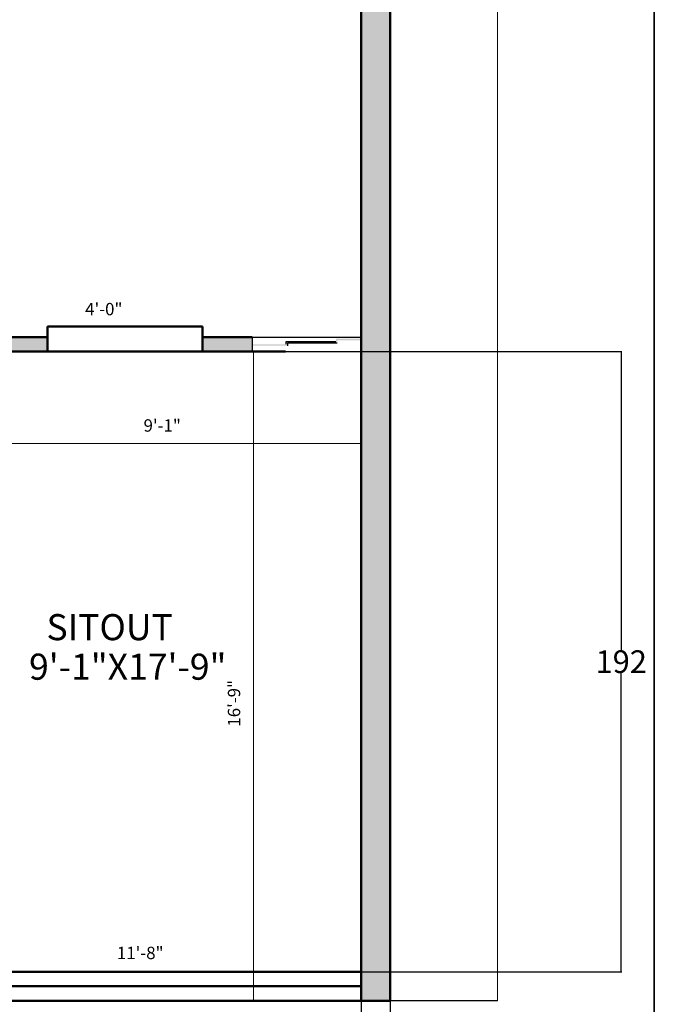
# Model space of a CAD drawing. Units: inches. Extents: x 1381 to 2246, y 1317 to 2168.
# Tile 12 of 15: x 2048 to 2244, y 1471 to 1776. Entities that reach past the tile are written whole.
import ezdxf

# ---------------------------------------------------------------- set-up
doc = ezdxf.new("R2010")
doc.units = ezdxf.units.IN
doc.header["$MEASUREMENT"] = 0
for name, color, linetype, lineweight in [('A-ANNO-DIMS', 2, 'Continuous', 18), ('A-ANNO-TEXT', 7, 'Continuous', 18), ('A-ANNO-TTLB', 7, 'Continuous', 35), ('A-AREA-IDEN', 3, 'Continuous', 25), ('A-GLAZ', 4, 'Continuous', 25), ('A-WALL', 7, 'Continuous', 50), ('A-WALL-PATT', 8, 'Continuous', 13)]:
    doc.layers.add(name, color=color, linetype=linetype, lineweight=lineweight)
doc.styles.get("Standard").update_dxf_attribs({"font": 'arial.ttf'})
doc.dimstyles.get("Standard").update_dxf_attribs({"dimtxt": 7, "dimasz": 0.18, "dimexe": 0.18, "dimexo": 0.0625, "dimgap": 0.09, "dimtad": 0, "dimtih": 1, "dimtoh": 1, "dimdec": 1, "dimzin": 0, "dimdsep": 46, "dimlunit": 3, "dimtxsty": 'Standard', "dimcen": 0.09, "dimadec": 0, "dimazin": 0, "dimtfac": 1, "dimtdec": 1, "dimtofl": 0, "dimtmove": 0, "dimatfit": 3, "dimfxl": 1, "dimtolj": 1, "dimtzin": 0, "dimarcsym": 0})

# ---------------------------------------------------------------- blocks, each defined once
blk = doc.blocks.new('*D75')
at = {"layer": 'A-ANNO-DIMS', "color": 0, "lineweight": -2, "transparency": 16777216}
for p, q in [((1862.81, 1471.85), (1862.81, 1384.36)), ((2162.31, 1471.85), (2162.31, 1384.36)), ((1862.99, 1384.54), (2000.57, 1384.54)), ((2162.13, 1384.54), (2024.54, 1384.54))]:
    blk.add_line(p, q, dxfattribs=at)
at = {"layer": 'A-ANNO-DIMS', "color": 0, "transparency": 16777216}
for points in [[(1862.99, 1384.57), (1862.99, 1384.51), (1862.81, 1384.54)], [(2162.13, 1384.57), (2162.13, 1384.51), (2162.31, 1384.54)]]:
    blk.add_solid(points, dxfattribs=at)
at = {"layer": 'Defpoints', "color": 0, "transparency": 16777216}
for p in [(1862.81, 1471.92), (2162.31, 1471.92), (2162.31, 1384.54)]:
    blk.add_point(p, dxfattribs=at)
at = {"layer": 'A-ANNO-DIMS', "color": 0, "transparency": 16777216, "insert": (2012.56, 1384.54), "char_height": 7, "attachment_point": 5}
blk.add_mtext('\\A1;299.5', dxfattribs=at)
blk = doc.blocks.new('*D86')
at = {"layer": 'A-ANNO-DIMS', "color": 0, "lineweight": -2, "transparency": 16777216}
for p, q in [((2153.37, 1672.92), (2234.02, 1672.92)), ((2233.84, 1672.74), (2233.84, 1580.58)), ((2233.84, 1481.1), (2233.84, 1573.25)), ((2153.37, 1480.92), (2234.02, 1480.92))]:
    blk.add_line(p, q, dxfattribs=at)
at = {"layer": 'A-ANNO-DIMS', "color": 0, "transparency": 16777216}
for points in [[(2233.81, 1672.74), (2233.87, 1672.74), (2233.84, 1672.92)], [(2233.81, 1481.1), (2233.87, 1481.1), (2233.84, 1480.92)]]:
    blk.add_solid(points, dxfattribs=at)
at = {"layer": 'Defpoints', "color": 0, "transparency": 16777216}
for p in [(2153.31, 1672.92), (2233.84, 1672.92), (2153.31, 1480.92)]:
    blk.add_point(p, dxfattribs=at)
at = {"layer": 'A-ANNO-DIMS', "color": 0, "transparency": 16777216, "insert": (2233.84, 1576.92), "char_height": 7, "attachment_point": 5}
blk.add_mtext('\\A1;192', dxfattribs=at)
blk = doc.blocks.new('*D91')
at = {"layer": 'A-ANNO-DIMS', "color": 0, "lineweight": -2, "transparency": 16777216}
for p, q in [((2012.56, 1471.85), (2012.56, 1384.36)), ((2153.31, 1471.85), (2153.31, 1384.36)), ((2012.74, 1384.54), (2068.61, 1384.54)), ((2153.13, 1384.54), (2097.25, 1384.54))]:
    blk.add_line(p, q, dxfattribs=at)
at = {"layer": 'A-ANNO-DIMS', "color": 0, "transparency": 16777216}
for points in [[(2012.74, 1384.57), (2012.74, 1384.51), (2012.56, 1384.54)], [(2153.13, 1384.57), (2153.13, 1384.51), (2153.31, 1384.54)]]:
    blk.add_solid(points, dxfattribs=at)
at = {"layer": 'Defpoints', "color": 0, "transparency": 16777216}
for p in [(2012.56, 1471.92), (2153.31, 1471.92), (2153.31, 1384.54)]:
    blk.add_point(p, dxfattribs=at)
at = {"layer": 'A-ANNO-DIMS', "color": 0, "transparency": 16777216, "insert": (2082.93, 1384.54), "char_height": 7, "attachment_point": 5}
blk.add_mtext('\\A1;140.75', dxfattribs=at)

msp = doc.modelspace()

# ---------------------------------------------------------------- hatches: boundary and pattern name
at = {"layer": 'A-GLAZ'}
h = msp.add_hatch(color=256, dxfattribs=at)
h.dxf.hatch_style = 1
h.paths.add_polyline_path([(2130.6579, 1675.6607), (2145.9627, 1675.6607), (2145.9627, 1676.3635), (2153.3052, 1676.3635), (2153.3052, 1676.9597), (2145.5577, 1676.9597), (2145.5577, 1676.0866), (2130.125, 1676.0866), (2130.125, 1675.1663), (2119.6192, 1675.1663), (2119.6192, 1674.7024), (2130.6579, 1674.7024)])
at = {"layer": 'A-WALL-PATT'}
h = msp.add_hatch(color=256, dxfattribs=at)
h.dxf.hatch_style = 1
h.paths.add_polyline_path([(1990.4785, 1915.9163), (1929.807, 1915.9163), (1929.807, 1911.4163), (1990.4785, 1911.4163)], flags=17)
h.paths.add_polyline_path([(1900.7902, 1915.9163), (1871.8052, 1915.9163), (1871.8052, 1911.4163), (1900.7902, 1911.4163)], flags=17)
h.paths.add_polyline_path([(2043.2216, 1915.9163), (2038.3052, 1915.9163), (2038.3052, 2035.4163), (2098.0373, 2035.4163), (2098.0373, 2039.9163), (2033.8052, 2039.9163), (2033.8052, 1915.9163), (2028.7731, 1915.9163), (2028.7731, 1911.4163), (2043.2216, 1911.4163)], flags=17)
h.paths.add_polyline_path([(2153.3052, 1915.9163), (2085.2216, 1915.9163), (2085.2216, 1911.4163), (2153.3052, 1911.4163)], flags=17)
h.paths.add_polyline_path([(1935.508, 1911.4163), (1931.008, 1911.4163), (1931.008, 1779.4163), (1899.8394, 1779.4163), (1899.8394, 1774.9163), (1902.8052, 1774.9163), (1979.3052, 1774.9163), (1979.3052, 1770.3401), (1983.8052, 1770.3401), (1983.8052, 1779.4163), (1935.508, 1779.4163)], flags=17)
h.paths.add_polyline_path([(1871.8052, 2083.9163), (2153.3052, 2083.9163), (2153.3052, 2039.9163), (2141.7178, 2039.9163), (2141.7178, 2035.4163), (2153.3052, 2035.4163), (2153.3052, 1471.9163), (2162.3052, 1471.9163), (2162.3052, 2092.9163), (1862.8052, 2092.9163), (1862.8052, 1471.9163), (1904.4174, 1471.9163), (1904.4174, 1480.9163), (1871.8052, 1480.9163), (1871.8052, 1569.4163), (1964.2348, 1569.4163), (1964.2348, 1578.4163), (1871.8052, 1578.4163)])
h.paths.add_polyline_path([(1907.3052, 1729.193), (1902.8052, 1729.193), (1902.8052, 1714.9163), (1871.8052, 1714.9163), (1871.8052, 1710.4163), (1932.8736, 1710.4163), (1932.8736, 1714.9163), (1907.3052, 1714.9163)], flags=17)
h.paths.add_polyline_path([(2044.3052, 1644.4163), (2039.8052, 1644.4163), (2039.8052, 1618.2205), (2044.3052, 1618.2205)], flags=17)
h.paths.add_polyline_path([(2044.3052, 1581.7679), (2039.8052, 1581.7679), (2039.8052, 1578.4163), (2027.577, 1578.4163), (2027.577, 1569.4163), (2044.3052, 1569.4163)], flags=17)
h = msp.add_hatch(color=256, dxfattribs=at)
h.dxf.hatch_style = 1
h.paths.add_polyline_path([(1873.9195, 1779.4163), (1871.8052, 1779.4163), (1871.8052, 1774.9163), (1873.9195, 1774.9163)])
h.paths.add_polyline_path([(1983.8052, 1779.4163), (1935.508, 1779.4163), (1935.508, 1911.4163), (1931.008, 1911.4163), (1931.008, 1779.4163), (1899.8394, 1779.4163), (1899.8394, 1774.9163), (1902.8052, 1774.9163), (1979.3052, 1774.9163), (1979.3052, 1770.3401), (1983.8052, 1770.3401)])
h.paths.add_polyline_path([(1907.3052, 1774.9163), (1902.8052, 1774.9163), (1902.8052, 1755.1129), (1907.3052, 1755.1129)])
h.paths.add_polyline_path([(1983.8052, 1734.7997), (1979.3052, 1734.7997), (1979.3052, 1714.9163), (1973.3503, 1714.9163), (1973.3503, 1710.4163), (1983.8052, 1710.4163)])
h.paths.add_polyline_path([(2044.3052, 1732.454), (2039.8052, 1732.454), (2039.8052, 1716.0149), (2024.8052, 1716.0149), (2024.8052, 1710.4163), (2039.8052, 1710.4163), (2039.8052, 1644.4163), (2044.3052, 1644.4163)])
h.paths.add_polyline_path([(2056.2659, 1677.4163), (2044.3052, 1677.4163), (2044.3052, 1672.9163), (2056.2659, 1672.9163)])
h.paths.add_polyline_path([(2119.6192, 1677.4163), (2104.2659, 1677.4163), (2104.2659, 1672.9163), (2119.6192, 1672.9163)])
h.paths.add_polyline_path([(2012.5552, 1480.9163), (1952.401, 1480.9163), (1952.401, 1471.9163), (2012.5552, 1471.9163)])
h.paths.add_polyline_path([(1870.8149, 1834.6368), (1933.6567, 1834.6368), (1933.6567, 1847.0047), (1870.8149, 1847.0047)], flags=9)

# ---------------------------------------------------------------- linework, layer by layer
at = {"layer": 'A-ANNO-DIMS'}
for p, q in [((2195.5946, 2092.9163), (2195.5946, 1471.9163)), ((2120.0865, 1471.9163), (2120.0865, 1672.9163)), ((2039.8052, 1644.4163), (2153.3052, 1644.4163))]:
    msp.add_line(p, q, dxfattribs=at)
at = {"layer": 'A-ANNO-TTLB'}
msp.add_line((2244.072, 2167.8236), (2244.072, 1316.7761), dxfattribs=at)
at = {"layer": 'A-GLAZ'}
for p, q in [((2119.6192, 1677.4163), (2119.6192, 1672.9163)), ((2119.6192, 1677.4163), (2153.3052, 1677.4163)), ((2153.3052, 1672.9163), (2153.3052, 1677.4163)), ((2130.125, 1675.1663), (2130.125, 1676.0866)), ((2130.125, 1676.0866), (2145.5577, 1676.0866)), ((2130.6579, 1674.7024), (2130.6579, 1675.6607)), ((2130.6579, 1675.6607), (2145.9627, 1675.6607)), ((2119.6192, 1672.9163), (2153.3052, 1672.9163)), ((2195.5946, 1471.9163), (2162.3052, 1471.9163))]:
    msp.add_line(p, q, dxfattribs=at)
at = {"layer": 'A-WALL'}
for p, q in [((2162.3052, 2092.9163), (2162.3052, 1471.9163)), ((2153.3052, 2035.4163), (2153.3052, 1471.9163)), ((2056.2659, 1672.9163), (2056.2659, 1680.6861)), ((2056.2659, 1680.6861), (2104.2659, 1680.6861)), ((2104.2659, 1680.6861), (2104.2659, 1672.9163)), ((2044.3052, 1677.4163), (2056.2659, 1677.4163)), ((2104.2659, 1677.4163), (2119.6192, 1677.4163)), ((2044.3052, 1672.9163), (2129.9278, 1672.9163)), ((1871.8052, 1480.9163), (2153.3052, 1480.9163)), ((2012.5552, 1480.9163), (2153.3052, 1480.9163)), ((2153.3052, 1480.9163), (2153.3052, 1471.9163)), ((2012.5552, 1476.4163), (2153.3052, 1476.4163)), ((1862.8052, 1471.9163), (2162.3052, 1471.9163)), ((2153.3052, 1471.9163), (2012.5552, 1471.9163))]:
    msp.add_line(p, q, dxfattribs=at)

# ---------------------------------------------------------------- texts
at = {"layer": 'A-ANNO-TEXT'}
for s, p in [('4\'-0"', (2067.9384, 1684.1577)), ('9\'-1"', (2086.0202, 1648.1237)), ('11\'-8"', (2077.7577, 1484.8192))]:
    msp.add_text(s, height=3.83139, dxfattribs=at).set_placement(p)
msp.add_text('16\'-9"', height=3.83139, rotation=90, dxfattribs=at).set_placement((2115.9259, 1556.7937))
at = {"layer": 'A-AREA-IDEN'}
for s, height, p in [('SITOUT', 8.07451, (2055.9667, 1583.5597)), ('9\'-1"X17\'-9"', 8.074511, (2050.5727, 1571.3201))]:
    msp.add_text(s, height=height, dxfattribs=at).set_placement(p)

# ---------------------------------------------------------------- dimensions: what is measured, and where the dimension line sits
at = {"layer": 'A-ANNO-DIMS'}
dim = msp.add_linear_dim(base=(2233.8446, 1672.9163), p1=(2153.3052, 1480.9163), p2=(2153.3052, 1672.9163), angle=90, dimstyle='Standard', override={"dimdec": 0, "dimlfac": 1, "dimrnd": 0, "dimzin": 0, "dimdsep": 46, "dimlunit": 2}, dxfattribs=at)
dim.commit()
dim.dimension.update_dxf_attribs({"geometry": '*D86', "text_midpoint": (2233.8446, 1576.9163)})
for base, p1, p2, override, picture, middle in [((2162.3052, 1384.5407), (1862.8052, 1471.9163), (2162.3052, 1471.9163), {"dimdec": 1, "dimlfac": 1, "dimrnd": 0, "dimzin": 0, "dimdsep": 46, "dimlunit": 2}, '*D75', (2012.5552, 1384.5407)), ((2153.3052, 1384.5407), (2012.5552, 1471.9163), (2153.3052, 1471.9163), {"dimdec": 2, "dimlfac": 1, "dimrnd": 0, "dimzin": 0, "dimdsep": 46, "dimlunit": 2}, '*D91', (2082.9302, 1384.5407))]:
    dim = msp.add_linear_dim(base=base, p1=p1, p2=p2, dimstyle='Standard', override=override, dxfattribs=at)
    dim.commit()
    dim.dimension.update_dxf_attribs({"geometry": picture, "text_midpoint": middle})

doc.saveas('drawing.dxf')
